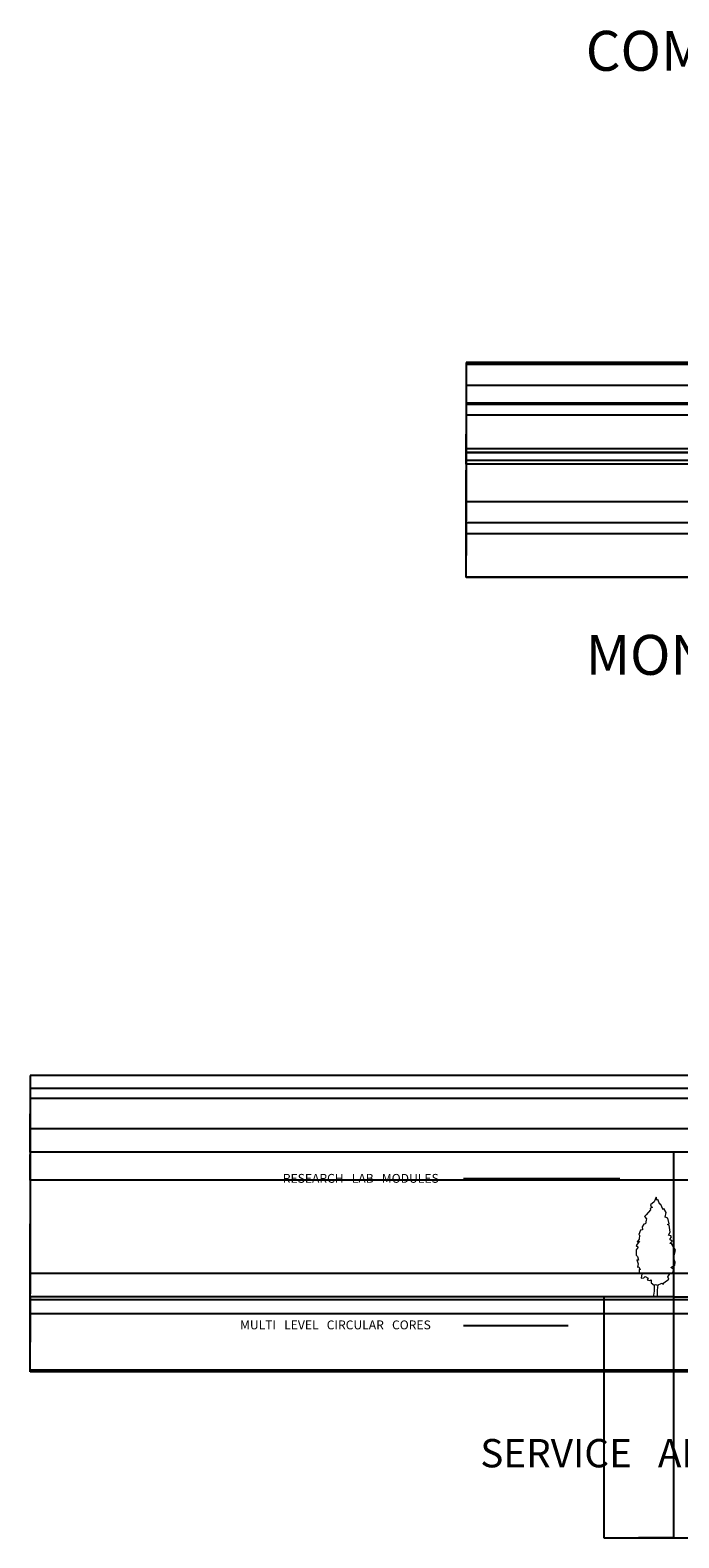
# Model space of a CAD drawing. Units: inches. Extents: x -32109 to 33221, y -19197 to 7608.
# Tile 1 of 25: x -32109 to -20585, y -19197 to 7608. Entities that reach past the tile are written whole.
import ezdxf

# ---------------------------------------------------------------- set-up
doc = ezdxf.new("R2010")
doc.units = ezdxf.units.IN
doc.header["$MEASUREMENT"] = 0
for name, color, linetype, lineweight in [('A-ANNO-DIMS', 2, 'Continuous', 18), ('A-ANNO-TEXT', 7, 'Continuous', 25), ('A-ELEV', 7, 'Continuous', 25), ('L-PLNT', 3, 'Continuous', 13)]:
    doc.layers.add(name, color=color, linetype=linetype, lineweight=lineweight)
doc.styles.get("Standard").update_dxf_attribs({"font": 'arial.ttf'})
doc.dimstyles.get("Standard").update_dxf_attribs({"dimtxt": 0.18, "dimasz": 0.18, "dimexe": 0.18, "dimexo": 0.0625, "dimgap": 0.09, "dimtad": 0, "dimtih": 1, "dimtoh": 1, "dimdec": 4, "dimzin": 0, "dimdsep": 46, "dimtxsty": 'Standard', "dimcen": 0.09, "dimadec": 0, "dimazin": 0, "dimtfac": 1, "dimtdec": 4, "dimtofl": 0, "dimtmove": 0, "dimatfit": 3, "dimfxl": 1, "dimtolj": 1, "dimtzin": 0, "dimarcsym": 0})

# ---------------------------------------------------------------- blocks, each defined once
blk = doc.blocks.new('*U2')
blk.add_lwpolyline([(-2.75400000000036, 191.699), (-6.7800000000002, 182.8509999999996), (-13.68200000000024, 176.9529999999995), (-11.95600000000013, 173.2659999999996), (-9.655999999999949, 172.529), (-14.25700000000006, 170.317), (-13.68200000000024, 167.3679999999999), (-21.73300000000017, 157.7829999999999), (-25.1840000000002, 154.8340000000003), (-21.15800000000036, 150.4099999999998), (-21.73300000000017, 147.4609999999998), (-22.88400000000001, 140.8249999999998), (-26.33400000000029, 140.087), (-29.21000000000004, 134.9259999999995), (-28.63499999999977, 129.0279999999998), (-32.66100000000006, 128.2909999999997), (-36.11099999999988, 120.1799999999998), (-34.38599999999997, 118.7059999999997), (-35.53600000000006, 111.3329999999996), (-38.98700000000008, 106.1709999999998), (-34.38599999999997, 107.6459999999997), (-40.71199999999999, 98.79799999999977), (-37.26099999999997, 95.8489999999997), (-40.71199999999999, 90.68799999999965), (-41.28700000000026, 80.36599999999999), (-38.41200000000026, 78.154), (-36.68600000000015, 70.78099999999995), (-39.5619999999999, 71.51799999999957), (-37.26099999999997, 64.14499999999998), (-38.41200000000026, 57.50899999999956), (-36.11099999999988, 58.24699999999984), (-33.23599999999988, 52.3479999999995), (-35.53600000000006, 53.08599999999978), (-34.96100000000024, 46.44999999999981), (-30.36000000000013, 44.9749999999999), (-31.50999999999977, 36.1279999999997), (-26.33400000000029, 36.86499999999978), (-23.45900000000029, 39.81399999999985), (-18.28300000000036, 36.1279999999997), (-20.00800000000027, 33.17799999999988), (-14.83199999999988, 31.70399999999972), (-11.95600000000013, 33.17799999999988), (-12.53099999999995, 27.27999999999975), (-6.204999999999927, 22.85599999999977), (-3.9050000000002, 24.33099999999968), (0.1209999999996398, 22.85599999999977), (8.172999999999774, 26.54299999999967), (11.62399999999979, 25.06799999999976), (12.19900000000007, 27.27999999999975), (21.40000000000009, 34.6529999999998), (19.67500000000018, 39.07699999999977), (23.70099999999957, 44.9749999999999), (30.02700000000004, 47.92399999999997), (30.60199999999986, 53.82299999999986), (25.42599999999993, 56.77199999999993), (32.90299999999979, 61.19599999999991), (34.05299999999988, 67.0939999999996), (30.60199999999986, 75.20499999999993), (34.6279999999997, 89.95100000000002), (26.57599999999957, 103.2219999999997), (23.70099999999957, 103.2219999999997), (28.30199999999968, 107.6459999999997), (23.70099999999957, 110.5949999999998), (26.57599999999957, 115.7559999999994), (25.42599999999993, 117.9679999999998), (20.82499999999982, 118.7059999999997), (24.27599999999984, 124.6040000000002), (22.55099999999993, 137.8759999999997), (19.09999999999991, 139.3499999999999), (22.55099999999993, 140.8249999999998), (19.67500000000018, 151.884), (14.49899999999979, 153.3589999999999), (16.22400000000016, 162.2069999999999), (12.19900000000007, 170.317), (10.47299999999995, 167.3679999999999), (5.871999999999843, 179.1649999999999), (4.146999999999934, 177.69), (0.6959999999999127, 187.2749999999996), (-0.4540000000001783, 185.7999999999997)], close=True)
for points in [[(-6.813000000000101, 23.66899999999987), (-6.813000000000101, 11.66899999999987), (-8.626999999999953, 0)], [(0.3869999999997162, 23.66899999999987), (-0.5760000000000219, 13.27099999999973), (-0.5760000000000219, 3.685999999999694), (0, 0)]]:
    blk.add_lwpolyline(points)
blk = doc.blocks.new('*D13')
at = {"layer": 'A-ANNO-DIMS', "color": 0, "lineweight": -2, "transparency": 16777216}
for p, q in [((-21916.328365, -16214.873241), (-21916.328365, -19197.348741)), ((5067.151383999999, -16244.175331), (5067.151383999999, -19197.348741)), ((-21916.148365, -19197.168741), (-8425.018722423602, -19197.168741)), ((5066.971383999999, -19197.168741), (-8424.158258576399, -19197.168741))]:
    blk.add_line(p, q, dxfattribs=at)
at = {"layer": 'A-ANNO-DIMS', "color": 0, "transparency": 16777216}
for points in [[(-21916.148365, -19197.138741), (-21916.148365, -19197.198741), (-21916.328365, -19197.168741)], [(5066.971383999999, -19197.138741), (5066.971383999999, -19197.198741), (5067.151383999999, -19197.168741)]]:
    blk.add_solid(points, dxfattribs=at)
at = {"layer": 'Defpoints', "color": 0, "transparency": 16777216}
for p in [(-21916.328365, -16214.810741), (5067.151383999999, -16244.112831), (5067.151383999999, -19197.168741)]:
    blk.add_point(p, dxfattribs=at)
at = {"layer": 'A-ANNO-DIMS', "color": 0, "transparency": 16777216, "insert": (-8424.5884905, -19197.168741), "char_height": 0.18, "attachment_point": 5}
blk.add_mtext('\\A1;26983', dxfattribs=at)
blk = doc.blocks.new('*D14')
at = {"layer": 'A-ANNO-DIMS', "color": 0, "lineweight": -2, "transparency": 16777216}
for p, q in [((-18893.90707200001, -10978.730223), (-32108.36667400003, -10978.73022300001)), ((-32108.18667400003, -10978.91022300001), (-32108.18667400003, -13611.23962386222)), ((-32108.18667400003, -16243.93283100001), (-32108.18667400003, -13611.6034301378)), ((5067.088884000002, -16244.11283100001), (-32108.36667400003, -16244.11283100001))]:
    blk.add_line(p, q, dxfattribs=at)
at = {"layer": 'A-ANNO-DIMS', "color": 0, "transparency": 16777216}
for points in [[(-32108.21667400003, -10978.91022300001), (-32108.15667400003, -10978.91022300001), (-32108.18667400003, -10978.73022300001)], [(-32108.21667400003, -16243.93283100001), (-32108.15667400003, -16243.93283100001), (-32108.18667400003, -16244.11283100001)]]:
    blk.add_solid(points, dxfattribs=at)
at = {"layer": 'Defpoints', "color": 0, "transparency": 16777216}
for p in [(-18893.84457200001, -10978.730223), (-32108.18667400003, -16244.11283100001), (5067.151384000002, -16244.11283100001)]:
    blk.add_point(p, dxfattribs=at)
at = {"layer": 'A-ANNO-DIMS', "color": 0, "transparency": 16777216, "insert": (-32108.18667400002, -13611.421527), "char_height": 0.18, "attachment_point": 5}
blk.add_mtext('\\A1;5265', dxfattribs=at)
blk = doc.blocks.new('*D21')
at = {"layer": 'A-ANNO-DIMS', "color": 0, "lineweight": -2, "transparency": 16777216}
for p, q in [((-5532.163600000002, -1149.229573), (-24361.99565300002, -1149.229573000003)), ((-24361.81565300002, -1149.409573000004), (-24361.81565300002, -1636.828167362214)), ((-24361.81565300002, -2124.610568000004), (-24361.81565300002, -1637.191973637794)), ((-5677.141660000002, -2124.790568000001), (-24361.99565300002, -2124.790568000003))]:
    blk.add_line(p, q, dxfattribs=at)
at = {"layer": 'A-ANNO-DIMS', "color": 0, "transparency": 16777216}
for points in [[(-24361.84565300001, -1149.409573000004), (-24361.78565300002, -1149.409573000004), (-24361.81565300002, -1149.229573000003)], [(-24361.84565300001, -2124.610568000004), (-24361.78565300002, -2124.610568000004), (-24361.81565300002, -2124.790568000003)]]:
    blk.add_solid(points, dxfattribs=at)
at = {"layer": 'Defpoints', "color": 0, "transparency": 16777216}
for p in [(-24361.81565300002, -1149.229573000003), (-5532.101100000001, -1149.229573), (-5677.079160000002, -2124.790568000001)]:
    blk.add_point(p, dxfattribs=at)
at = {"layer": 'A-ANNO-DIMS', "color": 0, "transparency": 16777216, "insert": (-24361.81565300001, -1637.010070499996), "char_height": 0.18, "attachment_point": 5}
blk.add_mtext('\\A1;975.6', dxfattribs=at)
blk = doc.blocks.new('*D23')
at = {"layer": 'A-ANNO-DIMS', "color": 0, "lineweight": -2, "transparency": 16777216}
for p, q in [((-4093.737957000001, -14968.07898000001), (-32108.36667400003, -14968.07898000001)), ((-32108.18667400003, -14968.25898000001), (-32108.18667400003, -15591.26295736222)), ((-32108.18667400003, -16214.63074100001), (-32108.18667400003, -15591.6267636378)), ((-4279.014689000002, -16214.810741), (-32108.36667400003, -16214.81074100001))]:
    blk.add_line(p, q, dxfattribs=at)
at = {"layer": 'A-ANNO-DIMS', "color": 0, "transparency": 16777216}
for points in [[(-32108.21667400003, -14968.25898000001), (-32108.15667400003, -14968.25898000001), (-32108.18667400003, -14968.07898000001)], [(-32108.21667400003, -16214.63074100001), (-32108.15667400003, -16214.63074100001), (-32108.18667400003, -16214.81074100001)]]:
    blk.add_solid(points, dxfattribs=at)
at = {"layer": 'Defpoints', "color": 0, "transparency": 16777216}
for p in [(-32108.18667400003, -14968.07898000001), (-4093.675457000002, -14968.07898000001), (-4278.952189000001, -16214.810741)]:
    blk.add_point(p, dxfattribs=at)
at = {"layer": 'A-ANNO-DIMS', "color": 0, "transparency": 16777216, "insert": (-32108.18667400002, -15591.4448605), "char_height": 0.18, "attachment_point": 5}
blk.add_mtext('\\A1;1246.7', dxfattribs=at)
blk = doc.blocks.new('*D35')
at = {"layer": 'A-ANNO-DIMS', "color": 0, "lineweight": -2, "transparency": 16777216}
for p, q in [((-18512.70931600001, -110.241638), (-24361.99565300002, -110.241638000001)), ((-24361.81565300002, -110.421638000001), (-24361.81565300002, -1117.334199862211)), ((-24361.81565300002, -2124.610568000002), (-24361.81565300002, -1117.698006137791)), ((-18512.70931600001, -2124.790568000001), (-24361.99565300002, -2124.790568000002))]:
    blk.add_line(p, q, dxfattribs=at)
at = {"layer": 'A-ANNO-DIMS', "color": 0, "transparency": 16777216}
for points in [[(-24361.84565300001, -110.421638000001), (-24361.78565300002, -110.421638000001), (-24361.81565300002, -110.241638000001)], [(-24361.84565300001, -2124.610568000002), (-24361.78565300002, -2124.610568000002), (-24361.81565300002, -2124.790568000002)]]:
    blk.add_solid(points, dxfattribs=at)
at = {"layer": 'Defpoints', "color": 0, "transparency": 16777216}
for p in [(-18512.64681600001, -110.241638), (-24361.81565300002, -2124.790568000002), (-18512.64681600001, -2124.790568000001)]:
    blk.add_point(p, dxfattribs=at)
at = {"layer": 'A-ANNO-DIMS', "color": 0, "transparency": 16777216, "insert": (-24361.81565300001, -1117.516102999994), "char_height": 0.18, "attachment_point": 5}
blk.add_mtext('\\A1;2014.5', dxfattribs=at)
blk = doc.blocks.new('*D36')
at = {"layer": 'A-ANNO-DIMS', "color": 0, "lineweight": -2, "transparency": 16777216}
for p, q in [((-17113.21748400001, 955.0880220000005), (-24361.99565300002, 955.0880219999992)), ((-24361.81565300002, 954.9080219999993), (-24361.81565300002, 422.6051565293307)), ((-24361.81565300002, -110.061638000001), (-24361.81565300002, 422.2412274706676)), ((-18512.70931600001, -110.241638), (-24361.99565300002, -110.241638000001))]:
    blk.add_line(p, q, dxfattribs=at)
at = {"layer": 'A-ANNO-DIMS', "color": 0, "transparency": 16777216}
for points in [[(-24361.84565300001, 954.9080219999993), (-24361.78565300002, 954.9080219999993), (-24361.81565300002, 955.0880219999992)], [(-24361.84565300001, -110.061638000001), (-24361.78565300002, -110.061638000001), (-24361.81565300002, -110.241638000001)]]:
    blk.add_solid(points, dxfattribs=at)
at = {"layer": 'Defpoints', "color": 0, "transparency": 16777216}
for p in [(-17113.15498400001, 955.0880220000005), (-24361.81565300002, -110.241638000001), (-18512.64681600001, -110.241638)]:
    blk.add_point(p, dxfattribs=at)
at = {"layer": 'A-ANNO-DIMS', "color": 0, "transparency": 16777216, "insert": (-24361.81565300001, 422.4231920000059), "char_height": 0.18, "attachment_point": 5}
blk.add_mtext('\\A1;1065.3', dxfattribs=at)
blk = doc.blocks.new('*D37')
at = {"layer": 'A-ANNO-DIMS', "color": 0, "lineweight": -2, "transparency": 16777216}
for p, q in [((-14538.09127400001, 1696.520148000001), (-24361.99565300002, 1696.520147999999)), ((-24361.81565300002, 1696.340147999999), (-24361.81565300002, -213.9532454706702)), ((-24361.81565300002, -2124.610568000003), (-24361.81565300002, -214.3171745293332)), ((-15192.66168600001, -2124.790568000001), (-24361.99565300002, -2124.790568000003))]:
    blk.add_line(p, q, dxfattribs=at)
at = {"layer": 'A-ANNO-DIMS', "color": 0, "transparency": 16777216}
for points in [[(-24361.84565300001, 1696.340147999999), (-24361.78565300002, 1696.340147999999), (-24361.81565300002, 1696.520147999999)], [(-24361.84565300001, -2124.610568000003), (-24361.78565300002, -2124.610568000003), (-24361.81565300002, -2124.790568000003)]]:
    blk.add_solid(points, dxfattribs=at)
at = {"layer": 'Defpoints', "color": 0, "transparency": 16777216}
for p in [(-14538.02877400001, 1696.520148000001), (-24361.81565300002, -2124.790568000003), (-15192.599186, -2124.790568000001)]:
    blk.add_point(p, dxfattribs=at)
at = {"layer": 'A-ANNO-DIMS', "color": 0, "transparency": 16777216, "insert": (-24361.81565300001, -214.1352099999948), "char_height": 0.18, "attachment_point": 5}
blk.add_mtext('\\A1;3821', dxfattribs=at)
blk = doc.blocks.new('*D38')
at = {"layer": 'A-ANNO-DIMS', "color": 0, "lineweight": -2, "transparency": 16777216}
for p, q in [((-11787.074272, -45.54407500000001), (-24361.99565300002, -45.54407500000204)), ((-24361.81565300002, -45.72407500000204), (-24361.81565300002, -1084.985418362212)), ((-24361.81565300002, -2124.610568000003), (-24361.81565300002, -1085.349224637792)), ((-11787.074272, -2124.790568000001), (-24361.99565300002, -2124.790568000003))]:
    blk.add_line(p, q, dxfattribs=at)
at = {"layer": 'A-ANNO-DIMS', "color": 0, "transparency": 16777216}
for points in [[(-24361.84565300001, -45.72407500000204), (-24361.78565300002, -45.72407500000204), (-24361.81565300002, -45.54407500000204)], [(-24361.84565300001, -2124.610568000003), (-24361.78565300002, -2124.610568000003), (-24361.81565300002, -2124.790568000003)]]:
    blk.add_solid(points, dxfattribs=at)
at = {"layer": 'Defpoints', "color": 0, "transparency": 16777216}
for p in [(-11787.011772, -45.54407500000001), (-24361.81565300002, -2124.790568000003), (-11787.011772, -2124.790568000001)]:
    blk.add_point(p, dxfattribs=at)
at = {"layer": 'A-ANNO-DIMS', "color": 0, "transparency": 16777216, "insert": (-24361.81565300001, -1085.167321499995), "char_height": 0.18, "attachment_point": 5}
blk.add_mtext('\\A1;2079.2', dxfattribs=at)
blk = doc.blocks.new('*D39')
at = {"layer": 'A-ANNO-DIMS', "color": 0, "lineweight": -2, "transparency": 16777216}
for p, q in [((-7375.940118000004, 1290.029218), (-24361.99565300002, 1290.029217999997)), ((-24361.81565300002, 1289.849217999998), (-24361.81565300002, -414.0189259706716)), ((-24361.81565300002, -2118.250999000004), (-24361.81565300002, -414.3828550293346)), ((-7754.474858000003, -2118.430999000001), (-24361.99565300002, -2118.430999000004))]:
    blk.add_line(p, q, dxfattribs=at)
at = {"layer": 'A-ANNO-DIMS', "color": 0, "transparency": 16777216}
for points in [[(-24361.84565300001, 1289.849217999998), (-24361.78565300002, 1289.849217999998), (-24361.81565300002, 1290.029217999997)], [(-24361.84565300001, -2118.250999000004), (-24361.78565300002, -2118.250999000004), (-24361.81565300002, -2118.430999000004)]]:
    blk.add_solid(points, dxfattribs=at)
at = {"layer": 'Defpoints', "color": 0, "transparency": 16777216}
for p in [(-7375.877618000004, 1290.029218), (-24361.81565300002, -2118.430999000004), (-7754.412358000003, -2118.430999000001)]:
    blk.add_point(p, dxfattribs=at)
at = {"layer": 'A-ANNO-DIMS', "color": 0, "transparency": 16777216, "insert": (-24361.81565300001, -414.2008904999961), "char_height": 0.18, "attachment_point": 5}
blk.add_mtext('\\A1;3408.5', dxfattribs=at)
blk = doc.blocks.new('*D40')
at = {"layer": 'A-ANNO-DIMS', "color": 0, "lineweight": -2, "transparency": 16777216}
for p, q in [((-5445.086779000002, 973.0114150000005), (-24361.99565300002, 973.0114149999976)), ((-24361.81565300002, 972.8314149999974), (-24361.81565300002, -575.7076119706716)), ((-24361.81565300002, -2124.610568000004), (-24361.81565300002, -576.0715410293345)), ((-5677.141660000002, -2124.790568000001), (-24361.99565300002, -2124.790568000003))]:
    blk.add_line(p, q, dxfattribs=at)
at = {"layer": 'A-ANNO-DIMS', "color": 0, "transparency": 16777216}
for points in [[(-24361.84565300001, 972.8314149999974), (-24361.78565300002, 972.8314149999974), (-24361.81565300002, 973.0114149999976)], [(-24361.84565300001, -2124.610568000004), (-24361.78565300002, -2124.610568000004), (-24361.81565300002, -2124.790568000003)]]:
    blk.add_solid(points, dxfattribs=at)
at = {"layer": 'Defpoints', "color": 0, "transparency": 16777216}
for p in [(-5445.024279000001, 973.0114150000005), (-24361.81565300002, -2124.790568000003), (-5677.079160000002, -2124.790568000001)]:
    blk.add_point(p, dxfattribs=at)
at = {"layer": 'A-ANNO-DIMS', "color": 0, "transparency": 16777216, "insert": (-24361.81565300001, -575.889576499996), "char_height": 0.18, "attachment_point": 5}
blk.add_mtext('\\A1;3098', dxfattribs=at)
blk = doc.blocks.new('*D41')
at = {"layer": 'A-ANNO-DIMS', "color": 0, "lineweight": -2, "transparency": 16777216}
for p, q in [((-651.0217760000003, 162.185712), (-24361.99565300002, 162.1857119999962)), ((-24361.81565300002, 162.0057119999962), (-24361.81565300002, -981.1205248622146)), ((-24361.81565300002, -2124.610568000005), (-24361.81565300002, -981.4843311377945)), ((-651.0217760000003, -2124.790568000001), (-24361.99565300002, -2124.790568000005))]:
    blk.add_line(p, q, dxfattribs=at)
at = {"layer": 'A-ANNO-DIMS', "color": 0, "transparency": 16777216}
for points in [[(-24361.84565300001, 162.0057119999962), (-24361.78565300002, 162.0057119999962), (-24361.81565300002, 162.1857119999962)], [(-24361.84565300001, -2124.610568000005), (-24361.78565300002, -2124.610568000005), (-24361.81565300002, -2124.790568000005)]]:
    blk.add_solid(points, dxfattribs=at)
at = {"layer": 'Defpoints', "color": 0, "transparency": 16777216}
for p in [(-650.9592760000002, 162.185712), (-24361.81565300002, -2124.790568000005), (-650.9592760000002, -2124.790568000001)]:
    blk.add_point(p, dxfattribs=at)
at = {"layer": 'A-ANNO-DIMS', "color": 0, "transparency": 16777216, "insert": (-24361.81565300001, -981.3024279999973), "char_height": 0.18, "attachment_point": 5}
blk.add_mtext('\\A1;2287', dxfattribs=at)
blk = doc.blocks.new('*D42')
at = {"layer": 'A-ANNO-DIMS', "color": 0, "lineweight": -2, "transparency": 16777216}
for p, q in [((-12501.42121900001, 764.1865930000002), (-24361.99565300002, 764.1865929999982)), ((-24361.81565300002, 764.0065929999982), (-24361.81565300002, 428.0747211377882)), ((-24361.81565300002, 91.77904299999811), (-24361.81565300002, 427.7109148622083)), ((-12488.224911, 91.59904300000002), (-24361.99565300002, 91.5990429999981))]:
    blk.add_line(p, q, dxfattribs=at)
at = {"layer": 'A-ANNO-DIMS', "color": 0, "transparency": 16777216}
for points in [[(-24361.84565300001, 764.0065929999982), (-24361.78565300002, 764.0065929999982), (-24361.81565300002, 764.1865929999982)], [(-24361.84565300001, 91.77904299999811), (-24361.78565300002, 91.77904299999811), (-24361.81565300002, 91.5990429999981)]]:
    blk.add_solid(points, dxfattribs=at)
at = {"layer": 'Defpoints', "color": 0, "transparency": 16777216}
for p in [(-12501.35871900001, 764.1865930000002), (-24361.81565300002, 91.5990429999981), (-12488.16241100001, 91.59904300000002)]:
    blk.add_point(p, dxfattribs=at)
at = {"layer": 'A-ANNO-DIMS', "color": 0, "transparency": 16777216, "insert": (-24361.81565300001, 427.892818000005), "char_height": 0.18, "attachment_point": 5}
blk.add_mtext('\\A1;672.6', dxfattribs=at)
blk = doc.blocks.new('*D43')
at = {"layer": 'A-ANNO-DIMS', "color": 0, "lineweight": -2, "transparency": 16777216}
for p, q in [((-7375.940118000004, 99.10345500000005), (-24361.99565300002, 99.10345499999731)), ((-24361.81565300002, 98.9234549999973), (-24361.81565300002, -1009.481868862213)), ((-24361.81565300002, -2118.250999000004), (-24361.81565300002, -1009.845675137793)), ((-7754.474858000003, -2118.430999000001), (-24361.99565300002, -2118.430999000004))]:
    blk.add_line(p, q, dxfattribs=at)
at = {"layer": 'A-ANNO-DIMS', "color": 0, "transparency": 16777216}
for points in [[(-24361.84565300001, 98.9234549999973), (-24361.78565300002, 98.9234549999973), (-24361.81565300002, 99.10345499999731)], [(-24361.84565300001, -2118.250999000004), (-24361.78565300002, -2118.250999000004), (-24361.81565300002, -2118.430999000004)]]:
    blk.add_solid(points, dxfattribs=at)
at = {"layer": 'Defpoints', "color": 0, "transparency": 16777216}
for p in [(-7375.877618000004, 99.10345500000005), (-24361.81565300002, -2118.430999000004), (-7754.412358000003, -2118.430999000001)]:
    blk.add_point(p, dxfattribs=at)
at = {"layer": 'A-ANNO-DIMS', "color": 0, "transparency": 16777216, "insert": (-24361.81565300001, -1009.663771999996), "char_height": 0.18, "attachment_point": 5}
blk.add_mtext('\\A1;2217.5', dxfattribs=at)
blk = doc.blocks.new('*D46')
at = {"layer": 'A-ANNO-DIMS', "color": 0, "lineweight": -2, "transparency": 16777216}
for p, q in [((-15626.56260400001, -780.5276970000004), (-24361.99565300002, -780.5276970000018)), ((-24361.81565300002, -780.7076970000016), (-24361.81565300002, -1062.24124897067)), ((-24361.81565300002, -1344.138730000002), (-24361.81565300002, -1062.605178029333)), ((-15626.56260400001, -1344.31873), (-24361.99565300002, -1344.318730000002))]:
    blk.add_line(p, q, dxfattribs=at)
at = {"layer": 'A-ANNO-DIMS', "color": 0, "transparency": 16777216}
for points in [[(-24361.84565300001, -780.7076970000016), (-24361.78565300002, -780.7076970000016), (-24361.81565300002, -780.5276970000018)], [(-24361.84565300001, -1344.138730000002), (-24361.78565300002, -1344.138730000002), (-24361.81565300002, -1344.318730000002)]]:
    blk.add_solid(points, dxfattribs=at)
at = {"layer": 'Defpoints', "color": 0, "transparency": 16777216}
for p in [(-15626.50010400001, -780.5276970000004), (-24361.81565300002, -1344.318730000002), (-15626.50010400001, -1344.31873)]:
    blk.add_point(p, dxfattribs=at)
at = {"layer": 'A-ANNO-DIMS', "color": 0, "transparency": 16777216, "insert": (-24361.81565300001, -1062.423213499994), "char_height": 0.18, "attachment_point": 5}
blk.add_mtext('\\A1;563.8', dxfattribs=at)
blk = doc.blocks.new('*D47')
at = {"layer": 'A-ANNO-DIMS', "color": 0, "lineweight": -2, "transparency": 16777216}
for p, q in [((-15626.56260400001, -1344.31873), (-24361.99565300002, -1344.318730000002)), ((-24361.81565300002, -1344.498730000002), (-24361.81565300002, -1734.372745862212)), ((-24361.81565300002, -2124.610568000003), (-24361.81565300002, -1734.736552137792)), ((-15909.136734, -2124.790568000001), (-24361.99565300002, -2124.790568000002))]:
    blk.add_line(p, q, dxfattribs=at)
at = {"layer": 'A-ANNO-DIMS', "color": 0, "transparency": 16777216}
for points in [[(-24361.84565300001, -1344.498730000002), (-24361.78565300002, -1344.498730000002), (-24361.81565300002, -1344.318730000002)], [(-24361.84565300001, -2124.610568000003), (-24361.78565300002, -2124.610568000003), (-24361.81565300002, -2124.790568000002)]]:
    blk.add_solid(points, dxfattribs=at)
at = {"layer": 'Defpoints', "color": 0, "transparency": 16777216}
for p in [(-15626.50010400001, -1344.31873), (-24361.81565300002, -2124.790568000002), (-15909.074234, -2124.790568000001)]:
    blk.add_point(p, dxfattribs=at)
at = {"layer": 'A-ANNO-DIMS', "color": 0, "transparency": 16777216, "insert": (-24361.81565300001, -1734.554648999995), "char_height": 0.18, "attachment_point": 5}
blk.add_mtext('\\A1;780.5', dxfattribs=at)
blk = doc.blocks.new('*D78')
at = {"layer": 'A-ANNO-DIMS', "color": 0, "lineweight": -2, "transparency": 16777216}
for p, q in [((-20682.344651, -12340.2456), (-20682.344651, -19197.348741)), ((-21916.328365, -16214.873241), (-21916.328365, -19197.348741)), ((-21916.148365, -19197.168741), (-21299.68643978718, -19197.168741)), ((-20682.524651, -19197.168741), (-21298.98657621283, -19197.168741))]:
    blk.add_line(p, q, dxfattribs=at)
at = {"layer": 'A-ANNO-DIMS', "color": 0, "transparency": 16777216}
for points in [[(-21916.148365, -19197.138741), (-21916.148365, -19197.198741), (-21916.328365, -19197.168741)], [(-20682.524651, -19197.138741), (-20682.524651, -19197.198741), (-20682.344651, -19197.168741)]]:
    blk.add_solid(points, dxfattribs=at)
at = {"layer": 'Defpoints', "color": 0, "transparency": 16777216}
for p in [(-20682.344651, -12340.1831), (-21916.328365, -16214.810741), (-20682.344651, -19197.168741)]:
    blk.add_point(p, dxfattribs=at)
at = {"layer": 'A-ANNO-DIMS', "color": 0, "transparency": 16777216, "insert": (-21299.336508, -19197.168741), "char_height": 0.18, "attachment_point": 5}
blk.add_mtext('\\A1;1234', dxfattribs=at)
blk = doc.blocks.new('*D79')
at = {"layer": 'A-ANNO-DIMS', "color": 0, "lineweight": -2, "transparency": 16777216}
for p, q in [((-20682.344651, -12340.2456), (-20682.344651, -19197.348741)), ((-17355.072806, -12340.2456), (-17355.072806, -19197.348741)), ((-20682.164651, -19197.168741), (-19019.06743927763, -19197.168741)), ((-17355.252806, -19197.168741), (-19018.35001772237, -19197.168741))]:
    blk.add_line(p, q, dxfattribs=at)
at = {"layer": 'A-ANNO-DIMS', "color": 0, "transparency": 16777216}
for points in [[(-20682.164651, -19197.138741), (-20682.164651, -19197.198741), (-20682.344651, -19197.168741)], [(-17355.252806, -19197.138741), (-17355.252806, -19197.198741), (-17355.072806, -19197.168741)]]:
    blk.add_solid(points, dxfattribs=at)
at = {"layer": 'Defpoints', "color": 0, "transparency": 16777216}
for p in [(-20682.344651, -12340.1831), (-17355.072806, -12340.1831), (-17355.072806, -19197.168741)]:
    blk.add_point(p, dxfattribs=at)
at = {"layer": 'A-ANNO-DIMS', "color": 0, "transparency": 16777216, "insert": (-19018.7087285, -19197.168741), "char_height": 0.18, "attachment_point": 5}
blk.add_mtext('\\A1;3327', dxfattribs=at)
blk = doc.blocks.new('*D84')
at = {"layer": 'A-ANNO-DIMS', "color": 0, "lineweight": -2, "transparency": 16777216}
for p, q in [((-21916.39086500001, -14914.70396400001), (-32108.36667400003, -14914.70396400001)), ((-32108.18667400003, -14914.88396400001), (-32108.18667400003, -15564.57538797068)), ((-32108.18667400003, -16214.63074100001), (-32108.18667400003, -15564.93931702934)), ((-21916.39086500001, -16214.810741), (-32108.36667400003, -16214.81074100001))]:
    blk.add_line(p, q, dxfattribs=at)
at = {"layer": 'A-ANNO-DIMS', "color": 0, "transparency": 16777216}
for points in [[(-32108.21667400003, -14914.88396400001), (-32108.15667400003, -14914.88396400001), (-32108.18667400003, -14914.70396400001)], [(-32108.21667400003, -16214.63074100001), (-32108.15667400003, -16214.63074100001), (-32108.18667400003, -16214.81074100001)]]:
    blk.add_solid(points, dxfattribs=at)
at = {"layer": 'Defpoints', "color": 0, "transparency": 16777216}
for p in [(-32108.18667400003, -14914.70396400001), (-21916.32836500001, -14914.70396400001), (-21916.32836500001, -16214.810741)]:
    blk.add_point(p, dxfattribs=at)
at = {"layer": 'A-ANNO-DIMS', "color": 0, "transparency": 16777216, "insert": (-32108.18667400002, -15564.75735249999), "char_height": 0.18, "attachment_point": 5}
blk.add_mtext('\\A1;1300', dxfattribs=at)
blk = doc.blocks.new('*D85')
at = {"layer": 'A-ANNO-DIMS', "color": 0, "lineweight": -2, "transparency": 16777216}
for p, q in [((-20682.40715100001, -12340.18310000001), (-32108.36667400003, -12340.18310000001)), ((-32108.18667400003, -12340.36310000001), (-32108.18667400003, -13627.26162886222)), ((-32108.18667400003, -14914.52396400001), (-32108.18667400003, -13627.6254351378)), ((-20682.40715100001, -14914.70396400001), (-32108.36667400003, -14914.70396400001))]:
    blk.add_line(p, q, dxfattribs=at)
at = {"layer": 'A-ANNO-DIMS', "color": 0, "transparency": 16777216}
for points in [[(-32108.21667400003, -12340.36310000001), (-32108.15667400003, -12340.36310000001), (-32108.18667400003, -12340.18310000001)], [(-32108.21667400003, -14914.52396400001), (-32108.15667400003, -14914.52396400001), (-32108.18667400003, -14914.70396400001)]]:
    blk.add_solid(points, dxfattribs=at)
at = {"layer": 'Defpoints', "color": 0, "transparency": 16777216}
for p in [(-20682.34465100001, -12340.18310000001), (-32108.18667400003, -14914.70396400001), (-20682.34465100001, -14914.70396400001)]:
    blk.add_point(p, dxfattribs=at)
at = {"layer": 'A-ANNO-DIMS', "color": 0, "transparency": 16777216, "insert": (-32108.18667400002, -13627.44353199999), "char_height": 0.18, "attachment_point": 5}
blk.add_mtext('\\A1;2574.5', dxfattribs=at)
blk = doc.blocks.new('*D86')
at = {"layer": 'A-ANNO-DIMS', "color": 0, "lineweight": -2, "transparency": 16777216}
for p, q in [((-18893.90707200001, -10978.730223), (-32108.36667400003, -10978.73022300001)), ((-32108.18667400003, -10978.91022300001), (-32108.18667400003, -11659.27469697068)), ((-32108.18667400003, -12340.00310000001), (-32108.18667400003, -11659.63862602934)), ((-17355.13530600001, -12340.18310000001), (-32108.36667400003, -12340.18310000001))]:
    blk.add_line(p, q, dxfattribs=at)
at = {"layer": 'A-ANNO-DIMS', "color": 0, "transparency": 16777216}
for points in [[(-32108.21667400003, -10978.91022300001), (-32108.15667400003, -10978.91022300001), (-32108.18667400003, -10978.73022300001)], [(-32108.21667400003, -12340.00310000001), (-32108.15667400003, -12340.00310000001), (-32108.18667400003, -12340.18310000001)]]:
    blk.add_solid(points, dxfattribs=at)
at = {"layer": 'Defpoints', "color": 0, "transparency": 16777216}
for p in [(-18893.84457200001, -10978.730223), (-32108.18667400003, -12340.18310000001), (-17355.07280600001, -12340.18310000001)]:
    blk.add_point(p, dxfattribs=at)
at = {"layer": 'A-ANNO-DIMS', "color": 0, "transparency": 16777216, "insert": (-32108.18667400002, -11659.4566615), "char_height": 0.18, "attachment_point": 5}
blk.add_mtext('\\A1;1361.5', dxfattribs=at)
blk = doc.blocks.new('*D87')
at = {"layer": 'A-ANNO-DIMS', "color": 0, "lineweight": -2, "transparency": 16777216}
for p, q in [((-16435.83369500001, -11210.746258), (-32108.36667400003, -11210.746258)), ((-32108.18667400003, -11210.926258), (-32108.18667400003, -13712.59659636222)), ((-32108.18667400003, -16214.63074100001), (-32108.18667400003, -13712.96040263779)), ((-16994.015761, -16214.810741), (-32108.36667400003, -16214.81074100001))]:
    blk.add_line(p, q, dxfattribs=at)
at = {"layer": 'A-ANNO-DIMS', "color": 0, "transparency": 16777216}
for points in [[(-32108.21667400003, -11210.926258), (-32108.15667400003, -11210.926258), (-32108.18667400003, -11210.746258)], [(-32108.21667400003, -16214.63074100001), (-32108.15667400003, -16214.63074100001), (-32108.18667400003, -16214.81074100001)]]:
    blk.add_solid(points, dxfattribs=at)
at = {"layer": 'Defpoints', "color": 0, "transparency": 16777216}
for p in [(-16435.77119500001, -11210.746258), (-32108.18667400003, -16214.81074100001), (-16993.95326100001, -16214.810741)]:
    blk.add_point(p, dxfattribs=at)
at = {"layer": 'A-ANNO-DIMS', "color": 0, "transparency": 16777216, "insert": (-32108.18667400002, -13712.77849949999), "char_height": 0.18, "attachment_point": 5}
blk.add_mtext('\\A1;5004', dxfattribs=at)
blk = doc.blocks.new('*D88')
at = {"layer": 'A-ANNO-DIMS', "color": 0, "lineweight": -2, "transparency": 16777216}
for p, q in [((-6450.017839000004, -11923.964476), (-32108.36667400003, -11923.964476)), ((-32108.18667400003, -11924.144476), (-32108.18667400003, -12380.67353997068)), ((-32108.18667400003, -12837.56653300001), (-32108.18667400003, -12381.03746902934)), ((-6450.017839000004, -12837.746533), (-32108.36667400003, -12837.74653300001))]:
    blk.add_line(p, q, dxfattribs=at)
at = {"layer": 'A-ANNO-DIMS', "color": 0, "transparency": 16777216}
for points in [[(-32108.21667400003, -11924.144476), (-32108.15667400003, -11924.144476), (-32108.18667400003, -11923.964476)], [(-32108.21667400003, -12837.56653300001), (-32108.15667400003, -12837.56653300001), (-32108.18667400003, -12837.74653300001)]]:
    blk.add_solid(points, dxfattribs=at)
at = {"layer": 'Defpoints', "color": 0, "transparency": 16777216}
for p in [(-6449.955339000005, -11923.964476), (-32108.18667400003, -12837.74653300001), (-6449.955339000005, -12837.746533)]:
    blk.add_point(p, dxfattribs=at)
at = {"layer": 'A-ANNO-DIMS', "color": 0, "transparency": 16777216, "insert": (-32108.18667400002, -12380.8555045), "char_height": 0.18, "attachment_point": 5}
blk.add_mtext('\\A1;913.8', dxfattribs=at)
blk = doc.blocks.new('*D89')
at = {"layer": 'A-ANNO-DIMS', "color": 0, "lineweight": -2, "transparency": 16777216}
for p, q in [((-13434.44544300001, -12837.746533), (-32108.36667400003, -12837.74653300001)), ((-32108.18667400003, -12837.92653300001), (-32108.18667400003, -14526.09667247068)), ((-32108.18667400003, -16214.63074100001), (-32108.18667400003, -14526.46060152934)), ((-12087.28817, -16214.810741), (-32108.36667400003, -16214.81074100001))]:
    blk.add_line(p, q, dxfattribs=at)
at = {"layer": 'A-ANNO-DIMS', "color": 0, "transparency": 16777216}
for points in [[(-32108.21667400003, -12837.92653300001), (-32108.15667400003, -12837.92653300001), (-32108.18667400003, -12837.74653300001)], [(-32108.21667400003, -16214.63074100001), (-32108.15667400003, -16214.63074100001), (-32108.18667400003, -16214.81074100001)]]:
    blk.add_solid(points, dxfattribs=at)
at = {"layer": 'Defpoints', "color": 0, "transparency": 16777216}
for p in [(-13434.38294300001, -12837.746533), (-32108.18667400003, -16214.81074100001), (-12087.22567, -16214.810741)]:
    blk.add_point(p, dxfattribs=at)
at = {"layer": 'A-ANNO-DIMS', "color": 0, "transparency": 16777216, "insert": (-32108.18667400002, -14526.278637), "char_height": 0.18, "attachment_point": 5}
blk.add_mtext('\\A1;3377', dxfattribs=at)
blk = doc.blocks.new('*D90')
at = {"layer": 'A-ANNO-DIMS', "color": 0, "lineweight": -2, "transparency": 16777216}
for p, q in [((-16994.015761, -14496.89128100001), (-32108.36667400003, -14496.89128100001)), ((-32108.18667400003, -14497.07128100001), (-32108.18667400003, -14856.96167986222)), ((-32108.18667400003, -15217.21588500001), (-32108.18667400003, -14857.32548613779)), ((-16994.015761, -15217.395885), (-32108.36667400003, -15217.39588500001))]:
    blk.add_line(p, q, dxfattribs=at)
at = {"layer": 'A-ANNO-DIMS', "color": 0, "transparency": 16777216}
for points in [[(-32108.21667400003, -14497.07128100001), (-32108.15667400003, -14497.07128100001), (-32108.18667400003, -14496.89128100001)], [(-32108.21667400003, -15217.21588500001), (-32108.15667400003, -15217.21588500001), (-32108.18667400003, -15217.39588500001)]]:
    blk.add_solid(points, dxfattribs=at)
at = {"layer": 'Defpoints', "color": 0, "transparency": 16777216}
for p in [(-16993.95326100001, -14496.89128100001), (-32108.18667400003, -15217.39588500001), (-16993.95326100001, -15217.395885)]:
    blk.add_point(p, dxfattribs=at)
at = {"layer": 'A-ANNO-DIMS', "color": 0, "transparency": 16777216, "insert": (-32108.18667400002, -14857.14358299999), "char_height": 0.18, "attachment_point": 5}
blk.add_mtext('\\A1;720.5', dxfattribs=at)
blk = doc.blocks.new('*D91')
at = {"layer": 'A-ANNO-DIMS', "color": 0, "lineweight": -2, "transparency": 16777216}
for p, q in [((-16994.015761, -15217.395885), (-32108.36667400003, -15217.39588500001)), ((-32108.18667400003, -15217.57588500001), (-32108.18667400003, -15715.92140986222)), ((-32108.18667400003, -16214.63074100001), (-32108.18667400003, -15716.2852161378)), ((-16994.015761, -16214.810741), (-32108.36667400003, -16214.81074100001))]:
    blk.add_line(p, q, dxfattribs=at)
at = {"layer": 'A-ANNO-DIMS', "color": 0, "transparency": 16777216}
for points in [[(-32108.21667400003, -15217.57588500001), (-32108.15667400003, -15217.57588500001), (-32108.18667400003, -15217.39588500001)], [(-32108.21667400003, -16214.63074100001), (-32108.15667400003, -16214.63074100001), (-32108.18667400003, -16214.81074100001)]]:
    blk.add_solid(points, dxfattribs=at)
at = {"layer": 'Defpoints', "color": 0, "transparency": 16777216}
for p in [(-16993.95326100001, -15217.395885), (-32108.18667400003, -16214.81074100001), (-16993.95326100001, -16214.810741)]:
    blk.add_point(p, dxfattribs=at)
at = {"layer": 'A-ANNO-DIMS', "color": 0, "transparency": 16777216, "insert": (-32108.18667400002, -15716.10331299999), "char_height": 0.18, "attachment_point": 5}
blk.add_mtext('\\A1;997.4', dxfattribs=at)
blk = doc.blocks.new('*D158')
at = {"layer": 'A-ANNO-DIMS', "color": 0, "lineweight": -2, "transparency": 16777216}
for p, q in [((5447.266114000002, 1662.169531000001), (-24361.99565300002, 1662.169530999996)), ((-24361.81565300002, 1661.989530999996), (-24361.81565300002, -230.1077594706735)), ((-24361.81565300002, -2122.568979000006), (-24361.81565300002, -230.4716885293365)), ((5279.201554000002, -2122.748979000001), (-24361.99565300002, -2122.748979000006))]:
    blk.add_line(p, q, dxfattribs=at)
at = {"layer": 'A-ANNO-DIMS', "color": 0, "transparency": 16777216}
for points in [[(-24361.84565300001, 1661.989530999996), (-24361.78565300002, 1661.989530999996), (-24361.81565300002, 1662.169530999996)], [(-24361.84565300001, -2122.568979000006), (-24361.78565300002, -2122.568979000006), (-24361.81565300002, -2122.748979000006)]]:
    blk.add_solid(points, dxfattribs=at)
at = {"layer": 'Defpoints', "color": 0, "transparency": 16777216}
for p in [(5447.328614000002, 1662.169531000001), (-24361.81565300002, -2122.748979000006), (5279.264054000002, -2122.748979000001)]:
    blk.add_point(p, dxfattribs=at)
at = {"layer": 'A-ANNO-DIMS', "color": 0, "transparency": 16777216, "insert": (-24361.81565300001, -230.289723999998), "char_height": 0.18, "attachment_point": 5}
blk.add_mtext('\\A1;3784.9', dxfattribs=at)
blk = doc.blocks.new('*D159')
at = {"layer": 'A-ANNO-DIMS', "color": 0, "lineweight": -2, "transparency": 16777216}
for p, q in [((-6094.734242000003, -11386.25619), (-32108.36667400003, -11386.25619000001)), ((-32108.18667400003, -11386.43619000001), (-32108.18667400003, -13800.35156236222)), ((-32108.18667400003, -16214.63074100001), (-32108.18667400003, -13800.7153686378)), ((-6952.836375000003, -16214.810741), (-32108.36667400003, -16214.81074100001))]:
    blk.add_line(p, q, dxfattribs=at)
at = {"layer": 'A-ANNO-DIMS', "color": 0, "transparency": 16777216}
for points in [[(-32108.21667400003, -11386.43619000001), (-32108.15667400003, -11386.43619000001), (-32108.18667400003, -11386.25619000001)], [(-32108.21667400003, -16214.63074100001), (-32108.15667400003, -16214.63074100001), (-32108.18667400003, -16214.81074100001)]]:
    blk.add_solid(points, dxfattribs=at)
at = {"layer": 'Defpoints', "color": 0, "transparency": 16777216}
for p in [(-6094.671742000002, -11386.25619), (-32108.18667400003, -16214.81074100001), (-6952.773875000004, -16214.810741)]:
    blk.add_point(p, dxfattribs=at)
at = {"layer": 'A-ANNO-DIMS', "color": 0, "transparency": 16777216, "insert": (-32108.18667400002, -13800.5334655), "char_height": 0.18, "attachment_point": 5}
blk.add_mtext('\\A1;4828.6', dxfattribs=at)

msp = doc.modelspace()

# ---------------------------------------------------------------- linework, layer by layer
at = {"layer": 'A-ELEV'}
for p, q in [((-18512.64681618521, -2124.790568085177), (-21911.81565297427, -2124.790568085177)), ((-18893.84457171501, -12340.18310009528), (-20682.34465069239, -12340.18310009528)), ((-20682.34465069239, -12340.18310009528), (-20682.34465069239, -14018.54332572247)), ((-21632.18850888475, -12813.54336576409), (-24412.25934011899, -12813.54336576409)), ((-20682.34465069239, -14365.148680594), (-20682.34465069239, -14914.70396449454)), ((-20682.34465069239, -14914.70396449454), (-21916.32836543051, -14914.70396449454)), ((-21916.32836543051, -14914.70396449454), (-21916.32836543051, -16214.8107410869)), ((-20682.34465069239, -14914.70396449454), (-16993.95326078703, -14914.70396449454)), ((-22549.88121455228, -15428.53474828426), (-24412.25934011899, -15428.53474828426)), ((-24194.61444585808, -16214.8107410869), (-30218.18667383001, -16214.8107410869)), ((-16993.95326078701, -16214.8107410869), (-24194.61444585808, -16214.8107410869))]:
    msp.add_line(p, q, dxfattribs=at)

# ---------------------------------------------------------------- block references
at = {"layer": 'L-PLNT', "xscale": 9.261495960754324, "yscale": 9.261495960754324, "zscale": 9.261495960754324}
msp.add_blockref('*U2', (-20962.98473697028, -14917.66104679439), dxfattribs=at)

# ---------------------------------------------------------------- texts
at = {"layer": 'A-ANNO-TEXT'}
for s, height, p in [('COMPREHENSIVE   ARCHITECTURAL   INTERLOCKING    CUBE   MEGA   CAMPUC   MASTER   PLAN ', 709.7949465747753, (-22238.10681632875, 6885.298304043546)), ('MONUMENTAL    FRONT   FACADE    ( CONCEPTUAL ONLY   NO DIMENSIONS )', 709.7949465747753, (-22238.10681632875, -3853.851877923695)), ('RESEARCH   LAB   MODULES', 157.8985042017455, (-27620.66816646535, -12885.26976966882)), ('MULTI   LEVEL   CIRCULAR   CORES', 157.8985042017455, (-28380.42375205315, -15490.44720386239)), ('SERVICE   AND   MECHNICAL  SPINE   REAR   PROFIL  ', 504.218310670369, (-24112.83023640446, -17944.24287726622))]:
    msp.add_text(s, height=height, dxfattribs=at).set_placement(p)

# ---------------------------------------------------------------- dimensions: what is measured, and where the dimension line sits
at = {"layer": 'A-ANNO-DIMS'}
for base, p1, p2, override, picture, middle in [((-24361.81565300002, -2122.748979000006), (5447.328613999999, 1662.169531), (5279.264054, -2122.748979), {"dimdec": 1, "dimlfac": 1, "dimrnd": 0, "dimzin": 0, "dimdsep": 46, "dimlunit": 2}, '*D158', (-24361.81565300001, -230.289723999998)), ((-24361.81565300002, -2124.790568000003), (-14538.028774, 1696.520148), (-15192.599186, -2124.790568), {"dimdec": 0, "dimlfac": 1, "dimrnd": 0, "dimzin": 0, "dimdsep": 46, "dimlunit": 2}, '*D37', (-24361.81565300001, -214.1352099999948)), ((-24361.81565300002, -2118.430999000004), (-7375.877618000001, 1290.029218), (-7754.412358, -2118.430999), {"dimdec": 1, "dimlfac": 1, "dimrnd": 0, "dimzin": 0, "dimdsep": 46, "dimlunit": 2}, '*D39', (-24361.81565300001, -414.2008904999961)), ((-24361.81565300002, -110.241638000001), (-17113.154984, 955.0880219999999), (-18512.646816, -110.241638), {"dimdec": 1, "dimlfac": 1, "dimrnd": 0, "dimzin": 0, "dimdsep": 46, "dimlunit": 2}, '*D36', (-24361.81565300001, 422.4231920000059)), ((-24361.81565300002, -2124.790568000003), (-5445.024279, 973.011415), (-5677.07916, -2124.790568), {"dimdec": 0, "dimlfac": 1, "dimrnd": 0, "dimzin": 0, "dimdsep": 46, "dimlunit": 2}, '*D40', (-24361.81565300001, -575.889576499996)), ((-24361.81565300002, 91.5990429999981), (-12501.358719, 764.186593), (-12488.162411, 91.599043), {"dimdec": 1, "dimlfac": 1, "dimrnd": 0, "dimzin": 0, "dimdsep": 46, "dimlunit": 2}, '*D42', (-24361.81565300001, 427.892818000005)), ((-24361.81565300002, -2118.430999000004), (-7375.877618000001, 99.103455), (-7754.412358, -2118.430999), {"dimdec": 1, "dimlfac": 1, "dimrnd": 0, "dimzin": 0, "dimdsep": 46, "dimlunit": 2}, '*D43', (-24361.81565300001, -1009.663771999996)), ((-24361.81565300002, -2124.790568000005), (-650.959276, 162.185712), (-650.959276, -2124.790568), {"dimdec": 0, "dimlfac": 1, "dimrnd": 0, "dimzin": 0, "dimdsep": 46, "dimlunit": 2}, '*D41', (-24361.81565300001, -981.3024279999973)), ((-24361.81565300002, -2124.790568000003), (-11787.011772, -45.54407499999999), (-11787.011772, -2124.790568), {"dimdec": 1, "dimlfac": 1, "dimrnd": 0, "dimzin": 0, "dimdsep": 46, "dimlunit": 2}, '*D38', (-24361.81565300001, -1085.167321499995)), ((-24361.81565300002, -2124.790568000002), (-18512.646816, -110.241638), (-18512.646816, -2124.790568), {"dimdec": 1, "dimlfac": 1, "dimrnd": 0, "dimzin": 0, "dimdsep": 46, "dimlunit": 2}, '*D35', (-24361.81565300001, -1117.516102999994)), ((-24361.81565300002, -1344.318730000002), (-15626.500104, -780.527697), (-15626.500104, -1344.31873), {"dimdec": 1, "dimlfac": 1, "dimrnd": 0, "dimzin": 0, "dimdsep": 46, "dimlunit": 2}, '*D46', (-24361.81565300001, -1062.423213499994)), ((-24361.81565300002, -1149.229573000003), (-5677.07916, -2124.790568), (-5532.1011, -1149.229573), {"dimdec": 1, "dimlfac": 1, "dimrnd": 0, "dimzin": 0, "dimdsep": 46, "dimlunit": 2}, '*D21', (-24361.81565300001, -1637.010070499996)), ((-24361.81565300002, -2124.790568000002), (-15626.500104, -1344.31873), (-15909.074234, -2124.790568), {"dimdec": 1, "dimlfac": 1, "dimrnd": 0, "dimzin": 0, "dimdsep": 46, "dimlunit": 2}, '*D47', (-24361.81565300001, -1734.554648999995)), ((-32108.18667400003, -12340.18310000001), (-18893.844572, -10978.730223), (-17355.072806, -12340.1831), {"dimdec": 1, "dimlfac": 1, "dimrnd": 0, "dimzin": 0, "dimdsep": 46, "dimlunit": 2}, '*D86', (-32108.18667400002, -11659.4566615)), ((-32108.18667400003, -16244.11283100001), (-18893.844572, -10978.730223), (5067.151383999999, -16244.112831), {"dimdec": 0, "dimlfac": 1, "dimrnd": 0, "dimzin": 0, "dimdsep": 46, "dimlunit": 2}, '*D14', (-32108.18667400002, -13611.421527)), ((-32108.18667400003, -16214.81074100001), (-16435.771195, -11210.746258), (-16993.953261, -16214.810741), {"dimdec": 0, "dimlfac": 1, "dimrnd": 0, "dimzin": 0, "dimdsep": 46, "dimlunit": 2}, '*D87', (-32108.18667400002, -13712.77849949999)), ((-32108.18667400003, -16214.81074100001), (-6094.671742, -11386.25619), (-6952.773875, -16214.810741), {"dimdec": 1, "dimlfac": 1, "dimrnd": 0, "dimzin": 0, "dimdsep": 46, "dimlunit": 2}, '*D159', (-32108.18667400002, -13800.5334655)), ((-32108.18667400003, -12837.74653300001), (-6449.955339, -11923.964476), (-6449.955339, -12837.746533), {"dimdec": 1, "dimlfac": 1, "dimrnd": 0, "dimzin": 0, "dimdsep": 46, "dimlunit": 2}, '*D88', (-32108.18667400002, -12380.8555045)), ((-32108.18667400003, -14914.70396400001), (-20682.344651, -12340.1831), (-20682.344651, -14914.703964), {"dimdec": 1, "dimlfac": 1, "dimrnd": 0, "dimzin": 0, "dimdsep": 46, "dimlunit": 2}, '*D85', (-32108.18667400002, -13627.44353199999)), ((-32108.18667400003, -16214.81074100001), (-13434.382943, -12837.746533), (-12087.22567, -16214.810741), {"dimdec": 0, "dimlfac": 1, "dimrnd": 0, "dimzin": 0, "dimdsep": 46, "dimlunit": 2}, '*D89', (-32108.18667400002, -14526.278637)), ((-32108.18667400003, -15217.39588500001), (-16993.953261, -14496.891281), (-16993.953261, -15217.395885), {"dimdec": 1, "dimlfac": 1, "dimrnd": 0, "dimzin": 0, "dimdsep": 46, "dimlunit": 2}, '*D90', (-32108.18667400002, -14857.14358299999)), ((-32108.18667400003, -14968.07898000001), (-4278.952188999999, -16214.810741), (-4093.675456999999, -14968.07898), {"dimdec": 1, "dimlfac": 1, "dimrnd": 0, "dimzin": 0, "dimdsep": 46, "dimlunit": 2}, '*D23', (-32108.18667400002, -15591.4448605)), ((-32108.18667400003, -14914.70396400001), (-21916.328365, -16214.810741), (-21916.328365, -14914.703964), {"dimdec": 0, "dimlfac": 1, "dimrnd": 0, "dimzin": 0, "dimdsep": 46, "dimlunit": 2}, '*D84', (-32108.18667400002, -15564.75735249999)), ((-32108.18667400003, -16214.81074100001), (-16993.953261, -15217.395885), (-16993.953261, -16214.810741), {"dimdec": 1, "dimlfac": 1, "dimrnd": 0, "dimzin": 0, "dimdsep": 46, "dimlunit": 2}, '*D91', (-32108.18667400002, -15716.10331299999))]:
    dim = msp.add_linear_dim(base=base, p1=p1, p2=p2, angle=90, dimstyle='Standard', override=override, dxfattribs=at)
    dim.commit()
    dim.dimension.update_dxf_attribs({"geometry": picture, "text_midpoint": middle})
for base, p1, p2, picture, middle in [((-20682.344651, -19197.168741), (-21916.328365, -16214.810741), (-20682.344651, -12340.1831), '*D78', (-21299.336508, -19197.168741)), ((-17355.072806, -19197.168741), (-20682.344651, -12340.1831), (-17355.072806, -12340.1831), '*D79', (-19018.7087285, -19197.168741)), ((5067.151383999999, -19197.168741), (-21916.328365, -16214.810741), (5067.151383999999, -16244.112831), '*D13', (-8424.5884905, -19197.168741))]:
    dim = msp.add_linear_dim(base=base, p1=p1, p2=p2, dimstyle='Standard', override={"dimdec": 0, "dimlfac": 1, "dimrnd": 0, "dimzin": 0, "dimdsep": 46, "dimlunit": 2}, dxfattribs=at)
    dim.commit()
    dim.dimension.update_dxf_attribs({"geometry": picture, "text_midpoint": middle})

doc.saveas('drawing.dxf')
